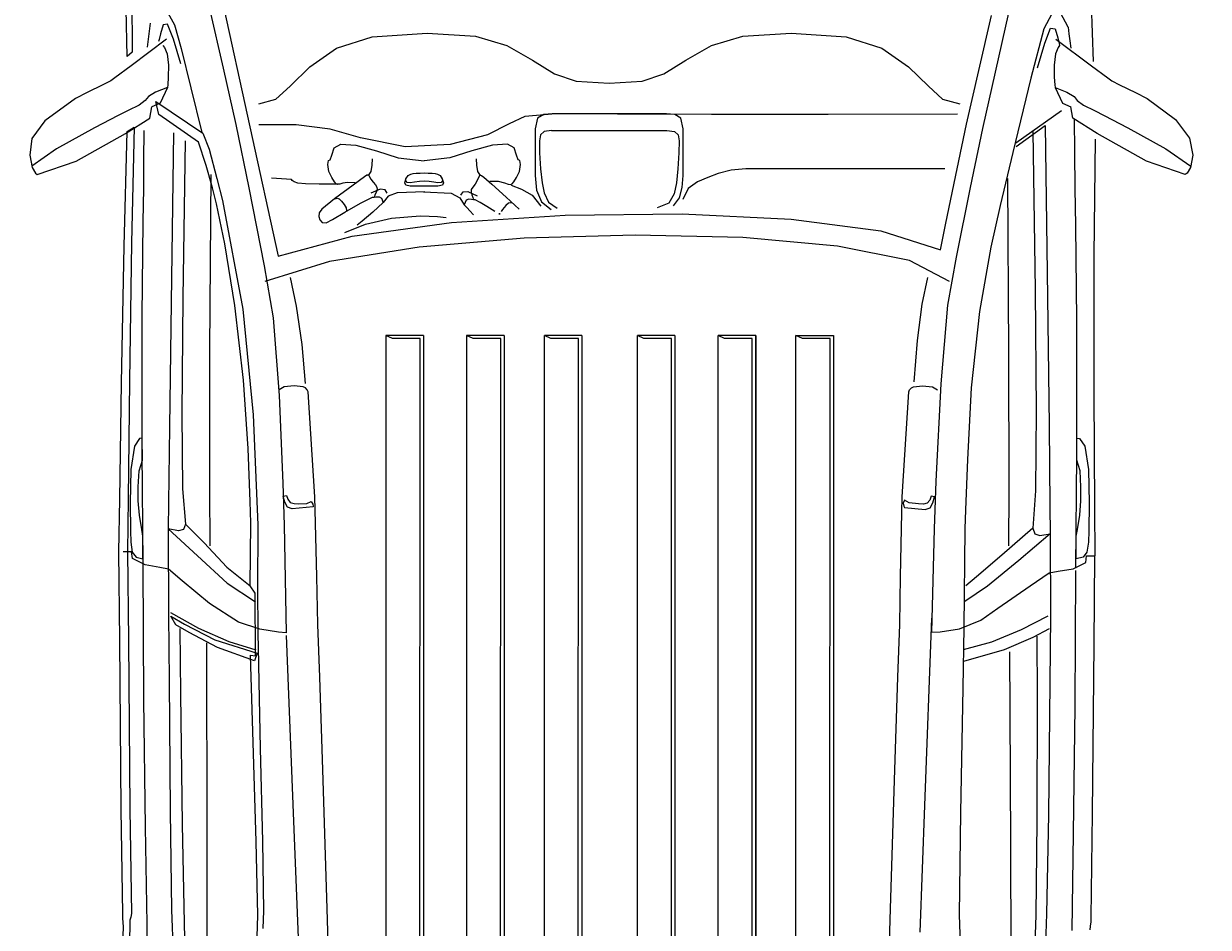
# Model space of a CAD drawing. Units: inches. Extents: x 37 to 706, y -568 to 110.
# Tile 4 of 24: x 126 to 171, y -413 to -378. Entities that reach past the tile are written whole.
import ezdxf

# ---------------------------------------------------------------- set-up
doc = ezdxf.new("R2010")
doc.units = ezdxf.units.IN
doc.header["$MEASUREMENT"] = 0
for name, color, linetype, lineweight in [('A-ANNO-DIMS', 2, 'Continuous', 18), ('A-SITE-VEHI', 8, 'Continuous', 13), ('A-WALL-PATT', 252, 'Continuous', 13)]:
    doc.layers.add(name, color=color, linetype=linetype, lineweight=lineweight)
doc.styles.get("Standard").update_dxf_attribs({"font": 'arial.ttf'})
doc.dimstyles.get("Standard").update_dxf_attribs({"dimtxt": 0.18, "dimasz": 0.18, "dimexe": 0.18, "dimexo": 0.0625, "dimgap": 0.09, "dimtad": 0, "dimtih": 1, "dimtoh": 1, "dimdec": 0, "dimzin": 0, "dimdsep": 46, "dimlunit": 3, "dimtxsty": 'Standard', "dimcen": 0.09, "dimadec": 0, "dimazin": 0, "dimtfac": 1, "dimtdec": 0, "dimtofl": 0, "dimtmove": 0, "dimatfit": 3, "dimfxl": 1, "dimtolj": 1, "dimtzin": 0, "dimarcsym": 0})

# ---------------------------------------------------------------- blocks, each defined once
blk = doc.blocks.new('CAR-SEDAN-PLAN')
for p, q in [((7.243, 63.902), (9.479, 53.69)), ((3.894, 63.679), (3.912, 61.483)), ((3.719, 61.318), (3.672, 63.126)), ((5.211, 63.093), (5.522, 62.522)), ((6.866, 63.136), (7.386, 60.866)), ((37.389, 62.984), (36.869, 60.714)), ((39.044, 62.941), (38.733, 62.37)), ((39.657, 62.441), (39.37, 62.983)), ((40.544, 63.318), (40.611, 61.119)), ((4.598, 62.593), (4.555, 62.29)), ((5.096, 62.522), (4.986, 62.183)), ((5.263, 62.546), (5.096, 62.522)), ((5.485, 61.977), (5.263, 62.546)), ((5.522, 62.522), (5.778, 61.618)), ((36.246, 60.784), (36.731, 62.877)), ((4.555, 62.29), (4.518, 61.981)), ((4.986, 62.183), (4.933, 61.962)), ((11.711, 61.631), (13.079, 62.064)), ((13.079, 62.064), (15.179, 62.211)), ((15.179, 62.211), (17.021, 62.087)), ((17.021, 62.087), (18.221, 61.732)), ((26.04, 61.732), (27.24, 62.087)), ((27.24, 62.087), (29.082, 62.211)), ((29.082, 62.211), (31.182, 62.064)), ((31.182, 62.064), (32.55, 61.631)), ((38.733, 62.37), (38.23, 60.486)), ((38.77, 61.826), (38.993, 62.394)), ((38.993, 62.394), (39.16, 62.37)), ((39.16, 62.37), (39.269, 62.031)), ((39.269, 62.031), (39.323, 61.81)), ((39.657, 62.441), (39.694, 62.178)), ((39.694, 62.178), (39.728, 61.911)), ((5.225, 61.98), (3.867, 60.965)), ((4.518, 61.981), (4.486, 61.667)), ((4.933, 61.962), (4.918, 61.883)), ((5.083, 61.731), (5.138, 61.656)), ((5.138, 61.656), (5.241, 61.415)), ((5.77, 61.03), (5.485, 61.977)), ((5.778, 61.618), (6.153, 60.123)), ((10.694, 60.923), (11.711, 61.631)), ((18.221, 61.732), (19.198, 61.17)), ((25.063, 61.17), (26.04, 61.732)), ((32.55, 61.631), (33.567, 60.923)), ((38.485, 60.879), (38.77, 61.826)), ((39.282, 61.656), (39.179, 61.415)), ((39.195, 61.98), (40.553, 60.965)), ((39.337, 61.731), (39.282, 61.656)), ((39.323, 61.81), (39.337, 61.731)), ((39.728, 61.911), (39.758, 61.639)), ((3.912, 61.483), (3.719, 61.318)), ((5.241, 61.415), (5.296, 60.985)), ((19.198, 61.17), (20.044, 60.65)), ((24.217, 60.65), (25.063, 61.17)), ((39.179, 61.415), (39.124, 60.985)), ((3.867, 60.965), (3.244, 60.496)), ((5.296, 60.985), (5.287, 60.527)), ((7.386, 60.866), (7.866, 58.722)), ((9.94, 60.179), (10.694, 60.923)), ((20.044, 60.65), (20.871, 60.374)), ((23.39, 60.374), (24.217, 60.65)), ((33.567, 60.923), (34.321, 60.179)), ((35.784, 58.735), (36.246, 60.784)), ((36.869, 60.714), (36.389, 58.57)), ((39.124, 60.985), (39.133, 60.527)), ((40.553, 60.965), (41.176, 60.496)), ((2.793, 60.236), (2.192, 59.94)), ((3.094, 60.381), (2.793, 60.236)), ((3.244, 60.496), (3.094, 60.381)), ((5.27, 60.235), (5.26, 60.133)), ((5.287, 60.527), (5.27, 60.235)), ((20.871, 60.374), (22.131, 60.293)), ((22.131, 60.293), (23.39, 60.374)), ((38.23, 60.486), (37.544, 57.648)), ((39.133, 60.527), (39.151, 60.235)), ((39.151, 60.235), (39.16, 60.133)), ((41.176, 60.496), (41.326, 60.381)), ((41.326, 60.381), (41.628, 60.236)), ((41.628, 60.236), (42.229, 59.941)), ((2.192, 59.94), (1.744, 59.706)), ((4.534, 59.788), (4.408, 59.635)), ((4.803, 59.956), (4.534, 59.788)), ((5.26, 60.133), (4.803, 59.956)), ((5.26, 60.133), (4.976, 59.529)), ((6.153, 60.123), (6.566, 58.409)), ((9.397, 59.68), (9.94, 60.179)), ((34.321, 60.179), (34.865, 59.68)), ((39.16, 60.133), (39.444, 59.529)), ((39.16, 60.133), (39.617, 59.956)), ((39.617, 59.956), (39.886, 59.788)), ((39.886, 59.788), (40.012, 59.635)), ((42.229, 59.941), (42.676, 59.706)), ((1.744, 59.706), (0.573, 58.863)), ((4.173, 59.456), (3.756, 59.246)), ((4.408, 59.635), (4.173, 59.456)), ((4.586, 58.96), (4.657, 59.387)), ((4.976, 59.529), (4.657, 59.387)), ((4.806, 59.598), (6.608, 58.388)), ((4.93, 59.103), (4.806, 59.598)), ((8.74, 59.507), (9.397, 59.68)), ((34.865, 59.68), (35.522, 59.507)), ((39.444, 59.529), (39.764, 59.387)), ((39.835, 58.96), (39.764, 59.387)), ((40.012, 59.635), (40.248, 59.456)), ((40.248, 59.456), (40.665, 59.246)), ((42.676, 59.706), (43.766, 58.903)), ((0.573, 58.863), (0.081, 58.181)), ((3.378, 59.067), (2.473, 58.595)), ((3.756, 59.246), (3.378, 59.067)), ((3.652, 58.378), (4.586, 58.96)), ((6.443, 58.044), (4.93, 59.103)), ((18.909, 59.028), (18.306, 58.744)), ((20.089, 59.124), (18.909, 59.028)), ((19.397, 58.963), (19.308, 58.556)), ((19.628, 59.105), (19.397, 58.963)), ((19.948, 59.122), (19.628, 59.105)), ((24.314, 59.122), (19.948, 59.122)), ((22.452, 59.111), (20.089, 59.124)), ((26.04, 59.104), (22.452, 59.111)), ((24.634, 59.105), (24.314, 59.122)), ((24.864, 58.963), (24.634, 59.105)), ((24.953, 58.556), (24.864, 58.963)), ((30.49, 59.105), (26.04, 59.104)), ((35.437, 59.117), (30.49, 59.105)), ((39.408, 59.245), (37.668, 58.002)), ((40.768, 58.378), (39.835, 58.96)), ((39.893, 58.942), (39.907, 57.649)), ((40.665, 59.246), (41.042, 59.067)), ((41.042, 59.067), (41.947, 58.595)), ((43.766, 58.903), (44.299, 58.201)), ((2.473, 58.595), (1.023, 57.787)), ((1.762, 57.317), (3.652, 58.378)), ((3.605, 54.068), (3.719, 58.456)), ((3.719, 58.456), (3.98, 58.613)), ((3.98, 58.613), (3.877, 54.201)), ((4.349, 58.487), (4.338, 57.349)), ((5.491, 58.398), (5.4, 51.914)), ((6.608, 58.388), (6.849, 57.774)), ((7.866, 58.722), (8.367, 56.297)), ((10.166, 58.704), (8.741, 58.704)), ((11.465, 58.539), (10.166, 58.704)), ((12.633, 58.209), (11.465, 58.539)), ((18.306, 58.744), (17.476, 58.319)), ((19.308, 58.556), (19.308, 56.766)), ((19.642, 58.446), (19.501, 58.322)), ((19.929, 58.483), (19.642, 58.446)), ((19.929, 58.483), (24.332, 58.483)), ((24.332, 58.483), (24.619, 58.446)), ((24.619, 58.446), (24.76, 58.322)), ((24.953, 56.766), (24.953, 58.556)), ((35.422, 57.018), (35.784, 58.735)), ((36.389, 58.57), (35.918, 56.312)), ((37.675, 57.879), (38.788, 58.684)), ((38.307, 58.463), (38.397, 52.383)), ((38.788, 58.684), (38.877, 52.125)), ((42.658, 57.317), (40.768, 58.378)), ((41.947, 58.595), (43.397, 57.787)), ((0.081, 58.181), (0, 57.551)), ((5.932, 58.096), (5.844, 52.097)), ((6.733, 57.156), (6.443, 58.044)), ((11.627, 57.82), (11.874, 57.964)), ((11.874, 57.964), (12.448, 57.926)), ((12.448, 57.926), (13.235, 57.705)), ((14.34, 57.866), (12.633, 58.209)), ((16.051, 57.949), (14.34, 57.866)), ((17.476, 58.319), (16.051, 57.949)), ((17.673, 57.926), (16.886, 57.705)), ((18.247, 57.964), (17.673, 57.926)), ((18.494, 57.82), (18.247, 57.964)), ((19.501, 58.322), (19.463, 58.09)), ((19.463, 58.09), (19.473, 57.639)), ((24.76, 58.322), (24.798, 58.09)), ((24.798, 58.09), (24.788, 57.639)), ((40.697, 58.154), (40.647, 53.716)), ((44.299, 58.201), (44.42, 57.551)), ((0, 57.551), (0.089, 57.074)), ((1.023, 57.787), (0.071, 57.125)), ((6.849, 57.774), (7.147, 56.658)), ((11.466, 57.369), (11.535, 57.542)), ((11.535, 57.542), (11.627, 57.82)), ((13.235, 57.705), (14.073, 57.447)), ((16.886, 57.705), (16.048, 57.447)), ((18.587, 57.542), (18.494, 57.82)), ((18.655, 57.369), (18.587, 57.542)), ((19.473, 57.639), (19.505, 57.028)), ((24.788, 57.639), (24.756, 57.028)), ((37.544, 57.648), (37.064, 55.622)), ((39.907, 57.649), (39.918, 56.282)), ((43.397, 57.787), (44.349, 57.125)), ((44.42, 57.551), (44.331, 57.074)), ((0.089, 57.074), (0.218, 56.857)), ((0.284, 56.806), (1.762, 57.317)), ((4.338, 57.349), (4.334, 56.285)), ((6.975, 56.299), (6.733, 57.156)), ((11.38, 57.195), (11.412, 57.338)), ((11.422, 56.921), (11.38, 57.195)), ((11.412, 57.338), (11.466, 57.369)), ((13.059, 57.159), (13.022, 56.924)), ((13.069, 57.405), (13.059, 57.159)), ((14.073, 57.447), (15.061, 57.323)), ((16.048, 57.447), (15.061, 57.323)), ((17.052, 57.405), (17.064, 57.16)), ((17.064, 57.16), (17.104, 56.925)), ((18.71, 57.338), (18.655, 57.369)), ((18.7, 56.921), (18.742, 57.195)), ((18.742, 57.195), (18.71, 57.338)), ((19.505, 57.028), (19.564, 56.492)), ((24.756, 57.028), (24.697, 56.492)), ((27.353, 57.026), (26.785, 56.971)), ((34.947, 57.026), (27.353, 57.026)), ((34.991, 54.942), (35.422, 57.018)), ((44.136, 56.806), (42.658, 57.317)), ((44.331, 57.074), (44.202, 56.857)), ((0.218, 56.857), (0.284, 56.806)), ((6.907, 56.804), (6.866, 50.096)), ((7.147, 56.658), (7.352, 55.813)), ((9.992, 56.613), (9.236, 56.668)), ((10.013, 56.583), (9.992, 56.613)), ((10.09, 56.523), (10.013, 56.583)), ((11.533, 56.687), (11.422, 56.921)), ((11.635, 56.528), (11.533, 56.687)), ((12.786, 56.72), (12.355, 56.402)), ((12.875, 56.778), (12.786, 56.72)), ((12.911, 56.779), (12.875, 56.778)), ((12.917, 56.768), (12.911, 56.779)), ((13.022, 56.924), (12.917, 56.768)), ((12.953, 56.766), (13.019, 56.626)), ((13.019, 56.626), (13.109, 56.514)), ((14.318, 56.49), (14.367, 56.638)), ((14.36, 56.563), (14.367, 56.638)), ((14.367, 56.638), (14.454, 56.763)), ((14.454, 56.763), (14.547, 56.817)), ((14.547, 56.817), (14.641, 56.839)), ((14.641, 56.839), (14.756, 56.854)), ((14.756, 56.854), (14.903, 56.863)), ((14.903, 56.863), (15.061, 56.866)), ((15.061, 56.866), (15.218, 56.863)), ((15.218, 56.863), (15.366, 56.854)), ((15.366, 56.854), (15.481, 56.839)), ((15.481, 56.839), (15.574, 56.817)), ((15.574, 56.817), (15.668, 56.763)), ((15.668, 56.763), (15.755, 56.638)), ((15.755, 56.638), (15.804, 56.49)), ((15.755, 56.638), (15.761, 56.563)), ((17.103, 56.601), (17.016, 56.44)), ((17.171, 56.766), (17.103, 56.601)), ((17.104, 56.925), (17.207, 56.766)), ((17.207, 56.766), (17.214, 56.776)), ((17.214, 56.776), (17.249, 56.774)), ((17.249, 56.774), (17.335, 56.711)), ((17.335, 56.711), (17.648, 56.433)), ((18.486, 56.528), (18.589, 56.687)), ((18.589, 56.687), (18.7, 56.921)), ((19.308, 56.766), (19.356, 56.213)), ((24.923, 56.308), (24.953, 56.766)), ((25.895, 56.696), (25.508, 56.53)), ((26.297, 56.842), (25.895, 56.696)), ((26.785, 56.971), (26.297, 56.842)), ((37.348, 56.652), (37.389, 49.984)), ((44.202, 56.857), (44.136, 56.806)), ((4.334, 56.285), (4.314, 54.993)), ((7.131, 55.691), (6.975, 56.299)), ((8.367, 56.297), (8.95, 53.318)), ((10.24, 56.475), (10.09, 56.523)), ((10.531, 56.453), (10.24, 56.475)), ((11.052, 56.441), (10.531, 56.453)), ((11.845, 56.437), (11.052, 56.441)), ((11.702, 56.448), (11.635, 56.528)), ((12.355, 56.402), (11.642, 55.878)), ((11.766, 56.42), (11.702, 56.448)), ((11.845, 56.437), (11.766, 56.42)), ((11.958, 56.473), (11.845, 56.437)), ((12.138, 56.495), (11.958, 56.473)), ((12.421, 56.483), (12.138, 56.495)), ((13.382, 56.251), (13.02, 56.096)), ((13.109, 56.514), (13.201, 56.416)), ((13.223, 56.122), (13.181, 56.026)), ((13.201, 56.416), (13.259, 56.323)), ((13.263, 56.228), (13.223, 56.122)), ((13.259, 56.323), (13.263, 56.228)), ((13.569, 56.226), (13.382, 56.251)), ((13.642, 56.091), (13.569, 56.226)), ((15.088, 56.145), (14.025, 56.105)), ((14.36, 56.396), (14.318, 56.49)), ((14.415, 56.496), (14.36, 56.563)), ((14.531, 56.364), (14.36, 56.396)), ((14.531, 56.483), (14.415, 56.496)), ((14.697, 56.511), (14.531, 56.483)), ((15.59, 56.364), (14.531, 56.364)), ((14.885, 56.536), (14.697, 56.511)), ((15.07, 56.547), (14.885, 56.536)), ((15.033, 56.145), (16.092, 56.088)), ((15.249, 56.536), (15.07, 56.547)), ((15.429, 56.511), (15.249, 56.536)), ((15.59, 56.483), (15.429, 56.511)), ((15.706, 56.496), (15.59, 56.483)), ((15.761, 56.396), (15.59, 56.364)), ((15.761, 56.563), (15.706, 56.496)), ((15.804, 56.49), (15.761, 56.396)), ((16.467, 56.017), (16.547, 56.148)), ((16.547, 56.148), (16.735, 56.163)), ((16.735, 56.163), (17.089, 55.989)), ((16.862, 56.228), (16.852, 56.134)), ((16.852, 56.134), (16.887, 56.026)), ((16.924, 56.318), (16.862, 56.228)), ((17.016, 56.44), (16.924, 56.318)), ((17.573, 56.556), (17.889, 56.549)), ((17.648, 56.433), (18.193, 55.945)), ((17.889, 56.549), (18.13, 56.492)), ((18.13, 56.492), (18.276, 56.437)), ((18.276, 56.437), (18.355, 56.42)), ((18.355, 56.42), (18.419, 56.448)), ((18.383, 56.393), (18.78, 56.247)), ((18.419, 56.448), (18.486, 56.528)), ((18.78, 56.247), (19.189, 56.016)), ((19.356, 56.213), (19.539, 55.764)), ((19.564, 56.492), (19.646, 56.107)), ((24.697, 56.492), (24.611, 56.07)), ((24.809, 55.915), (24.923, 56.308)), ((25.149, 56.27), (24.945, 55.856)), ((25.508, 56.53), (25.149, 56.27)), ((35.918, 56.312), (35.385, 53.644)), ((39.918, 56.282), (39.941, 54.841)), ((7.449, 54.154), (7.131, 55.691)), ((7.352, 55.813), (8.134, 51.663)), ((11.642, 55.878), (11.149, 55.48)), ((11.673, 55.883), (11.744, 55.903)), ((11.744, 55.903), (11.817, 55.879)), ((11.817, 55.879), (11.906, 55.788)), ((11.906, 55.788), (12.007, 55.658)), ((12.025, 55.371), (12.63, 55.707)), ((12.63, 55.707), (13.094, 55.946)), ((13.094, 55.946), (13.107, 55.941)), ((13.495, 55.733), (13.1, 55.373)), ((13.107, 55.941), (13.151, 55.937)), ((13.151, 55.937), (13.232, 55.948)), ((13.181, 56.026), (13.168, 55.97)), ((13.168, 55.97), (13.168, 55.951)), ((13.232, 55.948), (13.338, 55.959)), ((13.338, 55.959), (13.435, 55.908)), ((13.435, 55.908), (13.495, 55.733)), ((13.686, 55.974), (13.495, 55.733)), ((14.025, 56.105), (13.686, 55.974)), ((16.092, 56.088), (16.42, 55.921)), ((16.42, 55.921), (16.595, 55.651)), ((16.664, 55.823), (16.595, 55.651)), ((16.764, 55.869), (16.664, 55.823)), ((16.869, 55.852), (16.764, 55.869)), ((16.949, 55.838), (16.869, 55.852)), ((16.887, 56.026), (16.924, 55.928)), ((16.924, 55.928), (16.933, 55.871)), ((16.933, 55.871), (16.933, 55.852)), ((16.993, 55.84), (16.949, 55.838)), ((17.006, 55.843), (16.993, 55.84)), ((17.202, 55.734), (17.006, 55.843)), ((17.461, 55.581), (17.202, 55.734)), ((18.279, 55.71), (18.185, 55.624)), ((18.193, 55.945), (18.694, 55.483)), ((18.352, 55.729), (18.279, 55.71)), ((18.422, 55.706), (18.352, 55.729)), ((19.189, 56.016), (19.512, 55.595)), ((19.539, 55.764), (19.916, 55.467)), ((19.646, 56.107), (19.813, 55.756)), ((19.813, 55.756), (20.146, 55.524)), ((24.411, 55.715), (23.966, 55.531)), ((24.611, 56.07), (24.411, 55.715)), ((24.58, 55.614), (24.809, 55.915)), ((11.052, 55.336), (11.032, 55.197)), ((11.149, 55.48), (11.052, 55.336)), ((11.558, 55.084), (12.025, 55.371)), ((12.007, 55.658), (12.081, 55.535)), ((12.081, 55.535), (12.097, 55.422)), ((13.1, 55.373), (12.692, 55.023)), ((13.811, 55.137), (14.905, 55.222)), ((14.905, 55.222), (15.259, 55.221)), ((15.259, 55.221), (15.572, 55.208)), ((15.572, 55.208), (15.9, 55.17)), ((16.11, 54.971), (20.454, 55.259)), ((16.595, 55.651), (16.702, 55.534)), ((16.702, 55.534), (16.812, 55.413)), ((16.812, 55.413), (16.943, 55.271)), ((17.765, 55.393), (17.461, 55.581)), ((17.911, 55.307), (17.963, 55.31)), ((17.928, 55.308), (17.911, 55.307)), ((17.945, 55.309), (17.928, 55.308)), ((17.963, 55.31), (17.945, 55.309)), ((18.053, 55.468), (18.004, 55.394)), ((18.116, 55.545), (18.053, 55.468)), ((18.185, 55.624), (18.116, 55.545)), ((20.454, 55.259), (24.918, 55.306)), ((24.918, 55.306), (29.077, 55.104)), ((37.064, 55.622), (36.708, 54.03)), ((4.314, 54.993), (4.274, 51.392)), ((11.032, 55.197), (11.073, 55.073)), ((11.073, 55.073), (11.161, 54.978)), ((11.161, 54.978), (11.312, 54.961)), ((11.312, 54.961), (11.558, 55.084)), ((12.03, 54.597), (12.826, 54.914)), ((12.31, 54.446), (16.11, 54.971)), ((12.692, 55.023), (12.503, 54.866)), ((12.826, 54.914), (13.811, 55.137)), ((29.077, 55.104), (32.507, 54.649)), ((34.783, 53.934), (34.991, 54.942)), ((39.941, 54.841), (39.982, 51.24)), ((9.479, 53.69), (12.31, 54.446)), ((18.887, 54.369), (14.875, 54.03)), ((23.128, 54.492), (18.887, 54.369)), ((27.235, 54.394), (23.128, 54.492)), ((30.846, 54.07), (27.235, 54.394)), ((32.507, 54.649), (34.783, 53.934)), ((3.505, 48.842), (3.605, 54.068)), ((3.877, 54.201), (3.8, 48.921)), ((7.831, 51.803), (7.449, 54.154)), ((14.875, 54.03), (11.451, 53.479)), ((33.599, 53.515), (30.846, 54.07)), ((36.708, 54.03), (36.272, 51.578)), ((11.451, 53.479), (8.979, 52.723)), ((35.133, 52.723), (33.599, 53.515)), ((35.385, 53.644), (35.049, 51.82)), ((40.647, 53.716), (40.649, 48.459)), ((8.95, 53.318), (9.297, 51.325)), ((9.937, 52.871), (10.178, 51.78)), ((34.292, 52.871), (34.07, 51.849)), ((5.844, 52.097), (5.807, 47.67)), ((38.397, 52.383), (38.441, 47.777)), ((38.877, 52.125), (38.933, 47.216)), ((5.4, 51.914), (5.336, 47.171)), ((8.162, 48.95), (7.831, 51.803)), ((8.134, 51.663), (8.527, 47.62)), ((10.178, 51.78), (10.383, 50.312)), ((34.07, 51.849), (33.895, 50.463)), ((35.049, 51.82), (34.796, 48.812)), ((4.274, 51.392), (4.272, 47.831)), ((9.297, 51.325), (9.518, 48.368)), ((36.272, 51.578), (35.963, 48.661)), ((39.982, 51.24), (39.983, 47.679)), ((10.383, 50.312), (10.515, 48.827)), ((13.846, 50.543), (13.603, 50.661)), ((15.035, 50.661), (13.603, 50.661)), ((13.604, 13.133), (13.604, 50.661)), ((14.905, 50.543), (13.846, 50.543)), ((14.891, 13.73), (14.905, 50.543)), ((15.034, 50.661), (15.034, 13.133)), ((15.035, 50.661), (15.035, 13.133)), ((16.928, 50.543), (16.685, 50.661)), ((18.117, 50.661), (16.685, 50.661)), ((16.686, 13.133), (16.686, 50.661)), ((17.987, 50.543), (16.928, 50.543)), ((17.973, 13.73), (17.987, 50.543)), ((18.115, 50.661), (18.115, 13.133)), ((18.117, 50.661), (18.117, 13.133)), ((19.899, 50.543), (19.656, 50.661)), ((21.088, 50.661), (19.656, 50.661)), ((19.657, 13.133), (19.657, 50.661)), ((20.958, 50.543), (19.899, 50.543)), ((20.944, 13.73), (20.958, 50.543)), ((21.087, 50.661), (21.087, 13.133)), ((21.088, 50.661), (21.088, 13.133)), ((23.454, 50.543), (23.211, 50.661)), ((24.643, 50.661), (23.211, 50.661)), ((23.212, 13.133), (23.212, 50.661)), ((24.513, 50.543), (23.454, 50.543)), ((24.499, 13.73), (24.513, 50.543)), ((24.642, 50.661), (24.642, 13.133)), ((24.643, 50.661), (24.643, 13.133)), ((26.535, 50.543), (26.293, 50.661)), ((27.725, 50.661), (26.293, 50.661)), ((26.294, 13.133), (26.294, 50.661)), ((27.595, 50.543), (26.535, 50.543)), ((27.581, 13.73), (27.595, 50.543)), ((27.723, 50.661), (27.723, 13.133)), ((27.725, 50.661), (27.725, 13.133)), ((29.265, 13.133), (29.265, 50.661)), ((29.508, 50.543), (29.265, 50.661)), ((29.265, 50.661), (30.696, 50.661)), ((30.567, 50.543), (29.508, 50.543)), ((30.553, 13.73), (30.567, 50.543)), ((30.696, 50.661), (30.696, 13.133)), ((33.895, 50.463), (33.764, 48.882)), ((6.866, 50.096), (6.863, 44.784)), ((37.389, 49.984), (37.39, 44.744)), ((3.8, 48.921), (3.752, 44.431)), ((8.341, 46.338), (8.162, 48.95)), ((3.432, 44.406), (3.505, 48.842)), ((9.72, 48.689), (9.523, 48.579)), ((10.096, 48.73), (9.72, 48.689)), ((10.436, 48.697), (10.096, 48.73)), ((10.523, 48.654), (10.436, 48.697)), ((10.593, 48.583), (10.523, 48.654)), ((10.625, 48.497), (10.593, 48.583)), ((10.882, 44.496), (10.625, 48.497)), ((33.322, 44.496), (33.571, 48.497)), ((33.571, 48.497), (33.602, 48.583)), ((33.602, 48.583), (33.672, 48.654)), ((33.672, 48.654), (33.759, 48.697)), ((33.759, 48.697), (34.099, 48.73)), ((34.099, 48.73), (34.475, 48.689)), ((34.475, 48.689), (34.672, 48.579)), ((34.796, 48.812), (34.613, 45.086)), ((35.963, 48.661), (35.82, 45.919)), ((40.649, 48.459), (40.673, 44.07)), ((9.518, 48.368), (9.661, 45.012)), ((4.272, 47.831), (4.279, 46.22)), ((5.807, 47.67), (5.836, 44.794)), ((8.527, 47.62), (8.706, 43.417)), ((38.441, 47.777), (38.417, 44.723)), ((39.983, 47.679), (39.977, 46.068)), ((5.336, 47.171), (5.299, 44.26)), ((38.933, 47.216), (38.963, 44.139)), ((4.192, 46.715), (3.994, 46.427)), ((4.293, 46.735), (4.192, 46.715)), ((4.301, 45.897), (4.293, 46.735)), ((39.989, 45.897), (39.997, 46.735)), ((39.997, 46.735), (40.098, 46.715)), ((40.098, 46.715), (40.296, 46.427)), ((3.994, 46.427), (3.854, 45.534)), ((4.279, 46.22), (4.314, 41.922)), ((8.42, 44.315), (8.341, 46.338)), ((40.296, 46.427), (40.436, 45.534)), ((4.174, 45.486), (4.301, 45.897)), ((35.82, 45.919), (35.739, 43.991)), ((39.977, 46.068), (39.941, 41.77)), ((40.115, 45.486), (39.989, 45.897)), ((3.854, 45.534), (3.83, 44.25)), ((4.14, 44.879), (4.174, 45.486)), ((40.15, 44.879), (40.115, 45.486)), ((40.436, 45.534), (40.46, 44.25)), ((4.141, 44.332), (4.14, 44.879)), ((9.661, 45.012), (9.713, 43.414)), ((34.613, 45.086), (34.542, 43.262)), ((40.149, 44.332), (40.15, 44.879)), ((3.403, 42.392), (3.432, 44.406)), ((3.752, 44.431), (3.734, 42.392)), ((5.836, 44.794), (5.948, 43.449)), ((6.863, 44.784), (6.869, 42.622)), ((9.676, 44.516), (9.798, 44.542)), ((9.733, 44.29), (9.676, 44.516)), ((9.798, 44.542), (9.85, 44.396)), ((9.85, 44.396), (9.949, 44.274)), ((10.962, 41.449), (10.882, 44.496)), ((33.258, 41.449), (33.322, 44.496)), ((33.404, 44.362), (33.363, 44.248)), ((33.591, 44.267), (33.404, 44.362)), ((34.379, 44.368), (34.28, 44.247)), ((34.431, 44.514), (34.379, 44.368)), ((34.554, 44.489), (34.431, 44.514)), ((34.496, 44.262), (34.554, 44.489)), ((37.39, 44.744), (37.384, 42.623)), ((38.417, 44.723), (38.307, 43.297)), ((3.83, 44.25), (3.844, 43.196)), ((4.188, 43.792), (4.141, 44.332)), ((5.299, 44.26), (5.287, 43.269)), ((8.437, 43.503), (8.42, 44.315)), ((9.838, 44.098), (9.733, 44.29)), ((10.025, 44.031), (9.838, 44.098)), ((9.949, 44.274), (10.095, 44.234)), ((10.824, 44.11), (10.025, 44.031)), ((10.095, 44.234), (10.264, 44.226)), ((10.264, 44.226), (10.577, 44.234)), ((10.577, 44.234), (10.743, 44.307)), ((10.743, 44.307), (10.805, 44.214)), ((10.805, 44.214), (10.824, 44.14)), ((10.824, 44.14), (10.824, 44.11)), ((33.363, 44.248), (33.384, 44.134)), ((33.384, 44.134), (33.405, 44.082)), ((33.405, 44.082), (34.204, 44.004)), ((33.943, 44.22), (33.591, 44.267)), ((34.134, 44.207), (33.943, 44.22)), ((34.28, 44.247), (34.134, 44.207)), ((34.204, 44.004), (34.391, 44.071)), ((34.391, 44.071), (34.496, 44.262)), ((35.739, 43.991), (35.714, 43.262)), ((38.963, 44.139), (38.971, 43.074)), ((40.102, 43.792), (40.149, 44.332)), ((40.46, 44.25), (40.446, 43.196)), ((40.673, 44.07), (40.687, 42.232)), ((4.273, 43.24), (4.188, 43.792)), ((5.948, 43.449), (5.871, 43.237)), ((5.948, 43.449), (6.66, 42.737)), ((8.416, 41.085), (8.437, 43.503)), ((40.017, 43.24), (40.102, 43.792)), ((3.844, 43.196), (3.857, 42.759)), ((4.32, 42.987), (4.273, 43.24)), ((5.287, 43.269), (6.407, 42.232)), ((5.672, 43.197), (5.287, 43.269)), ((5.287, 43.269), (5.301, 39.967)), ((5.871, 43.237), (5.672, 43.197)), ((8.706, 43.417), (8.689, 40.947)), ((9.713, 43.414), (9.796, 39.289)), ((34.542, 43.262), (34.438, 39.318)), ((35.714, 43.262), (35.681, 39.496)), ((38.307, 43.297), (37.13, 42.261)), ((38.971, 43.074), (37.772, 42.057)), ((38.307, 43.297), (38.385, 43.074)), ((38.385, 43.074), (38.586, 43.013)), ((38.586, 43.013), (38.971, 43.074)), ((38.971, 43.074), (38.982, 39.925)), ((39.97, 42.987), (40.017, 43.24)), ((40.446, 43.196), (40.433, 42.759)), ((3.857, 42.759), (3.913, 42.374)), ((4.32, 42.116), (4.32, 42.987)), ((6.66, 42.737), (7.526, 41.803)), ((39.97, 42.116), (39.97, 42.987)), ((40.433, 42.759), (40.377, 42.374)), ((3.432, 39.004), (3.403, 42.392)), ((3.888, 42.384), (3.568, 42.392)), ((3.734, 42.392), (3.762, 39.007)), ((3.924, 42.135), (3.888, 42.384)), ((3.913, 42.374), (4.061, 42.185)), ((4.399, 41.888), (3.924, 42.135)), ((4.061, 42.185), (4.32, 42.116)), ((6.407, 42.232), (7.533, 41.191)), ((37.13, 42.261), (36.157, 41.433)), ((40.229, 42.185), (39.97, 42.116)), ((40.377, 42.374), (40.229, 42.185)), ((40.332, 41.983), (40.367, 42.232)), ((40.367, 42.232), (40.674, 42.232)), ((40.658, 38.847), (40.687, 42.232)), ((4.314, 41.922), (4.342, 36.731)), ((4.968, 41.787), (4.399, 41.888)), ((5.301, 41.728), (4.968, 41.787)), ((5.819, 41.275), (5.301, 41.728)), ((7.526, 41.803), (8.416, 41.085)), ((37.772, 42.057), (36.584, 41.081)), ((38.936, 41.591), (39.274, 41.645)), ((39.274, 41.645), (39.851, 41.74)), ((39.851, 41.74), (40.332, 41.983)), ((39.946, 41.674), (39.918, 36.482)), ((6.86, 40.42), (5.819, 41.275)), ((7.533, 41.191), (8.616, 40.477)), ((10.998, 39.61), (10.962, 41.449)), ((33.232, 39.61), (33.258, 41.449)), ((36.157, 41.433), (35.752, 41.094)), ((38.211, 41.09), (38.936, 41.591)), ((8.61, 40.812), (8.416, 41.085)), ((8.623, 38.413), (8.61, 40.812)), ((8.689, 40.947), (8.707, 39.376)), ((36.584, 41.081), (35.717, 40.49)), ((36.975, 40.234), (38.211, 41.09)), ((7.97, 39.706), (6.86, 40.42)), ((5.301, 39.967), (5.315, 37.467)), ((5.378, 40.068), (6.446, 39.47)), ((5.576, 39.596), (5.383, 39.926)), ((5.383, 39.926), (5.907, 39.624)), ((34.436, 39.852), (34.17, 32.694)), ((36.321, 39.78), (36.975, 40.234)), ((38.884, 39.936), (37.863, 39.414)), ((38.982, 39.925), (38.961, 37.396)), ((6.083, 39.306), (5.576, 39.596)), ((5.727, 39.459), (5.754, 36.963)), ((5.907, 39.624), (7.068, 39.031)), ((6.446, 39.47), (7.6, 38.961)), ((8.786, 39.439), (7.97, 39.706)), ((8.707, 39.376), (8.71, 39.215)), ((9.493, 39.318), (8.786, 39.439)), ((11.071, 37.604), (10.998, 39.61)), ((33.159, 37.604), (33.232, 39.61)), ((34.768, 39.333), (35.515, 39.45)), ((35.515, 39.45), (36.321, 39.78)), ((35.681, 39.496), (35.635, 37.18)), ((37.863, 39.414), (36.73, 38.932)), ((38.331, 39.125), (38.947, 39.462)), ((3.493, 32.542), (3.432, 39.004)), ((3.762, 39.007), (3.823, 32.551)), ((7.162, 38.735), (6.083, 39.306)), ((7.068, 39.031), (8.678, 38.516)), ((7.6, 38.961), (8.63, 38.647)), ((8.71, 39.215), (8.718, 38.766)), ((9.796, 39.289), (9.493, 39.318)), ((9.785, 39.195), (10.065, 32.102)), ((34.438, 39.318), (34.768, 39.333)), ((36.73, 38.932), (35.646, 38.643)), ((37.235, 38.651), (38.331, 39.125)), ((38.468, 39.17), (38.473, 36.823)), ((6.745, 38.908), (6.755, 31.469)), ((8.583, 38.221), (7.162, 38.735)), ((8.678, 38.516), (8.583, 38.221)), ((8.718, 38.766), (8.731, 38.071)), ((35.681, 38.217), (37.235, 38.651)), ((37.423, 38.564), (37.433, 36.292)), ((40.598, 32.392), (40.658, 38.847)), ((8.528, 35.109), (8.424, 38.44)), ((8.424, 38.44), (8.623, 38.413)), ((8.731, 38.071), (8.801, 34.877)), ((11.199, 33.662), (11.071, 37.604)), ((33.03, 33.662), (33.159, 37.604)), ((5.315, 37.467), (5.354, 32.465)), ((35.635, 37.18), (35.548, 32.425)), ((38.961, 37.396), (38.908, 32.341)), ((4.342, 36.731), (4.403, 31.875)), ((5.754, 36.963), (5.818, 31.97)), ((38.473, 36.823), (38.469, 32.105)), ((37.433, 36.292), (37.457, 31.221)), ((39.918, 36.482), (39.857, 31.627)), ((8.645, 31.317), (8.528, 35.109)), ((8.801, 34.877), (8.881, 31.335)), ((11.355, 28.753), (11.199, 33.662)), ((32.874, 28.753), (33.03, 33.662)), ((34.17, 32.694), (34.002, 27.855)), ((3.546, 28.561), (3.493, 32.542)), ((3.823, 32.551), (3.876, 28.574)), ((5.354, 32.465), (5.415, 28.71)), ((35.548, 32.425), (35.501, 28.522)), ((38.908, 32.341), (38.84, 28.558)), ((40.545, 28.416), (40.598, 32.392)), ((4.403, 31.875), (4.464, 28.172)), ((5.818, 31.97), (5.892, 28.219)), ((10.065, 32.102), (10.25, 27.635)), ((38.469, 32.105), (38.427, 28.503)), ((6.755, 31.469), (6.762, 26.153)), ((8.713, 28.508), (8.645, 31.317)), ((8.881, 31.335), (8.919, 28.667)), ((39.857, 31.627), (39.796, 27.924)), ((37.457, 31.221), (37.48, 25.971)), ((3.551, 28.393), (3.546, 28.561)), ((3.876, 28.574), (3.856, 28.436)), ((5.415, 28.71), (5.486, 26.554)), ((8.919, 28.667), (8.894, 27.992)), ((11.511, 23.847), (11.355, 28.753)), ((32.718, 23.847), (32.874, 28.753)), ((35.501, 28.522), (35.566, 26.682)), ((38.84, 28.558), (38.769, 26.402)), ((3.52, 26.505), (3.579, 28.059)), ((3.558, 28.225), (3.551, 28.393)), ((3.579, 28.059), (3.558, 28.225)), ((3.815, 28.178), (3.801, 27.531)), ((3.819, 28.315), (3.815, 28.178)), ((3.856, 28.436), (3.819, 28.315)), ((4.464, 28.172), (4.492, 26.437)), ((5.892, 28.219), (5.946, 25.954)), ((8.671, 27.267), (8.713, 28.508)), ((38.427, 28.503), (38.356, 26.347)), ((40.498, 27.951), (40.519, 28.091)), ((40.519, 28.091), (40.535, 28.246)), ((40.535, 28.246), (40.545, 28.416))]:
    blk.add_line(p, q)
blk = doc.blocks.new('*D29')
at = {"layer": 'A-ANNO-DIMS', "color": 0, "lineweight": -2, "transparency": 16777216}
for p, q in [((170.913, -348.62), (184.856, -348.62)), ((184.676, -348.8), (184.676, -394.522)), ((184.676, -440.609), (184.676, -394.888)), ((170.913, -440.789), (184.856, -440.789))]:
    blk.add_line(p, q, dxfattribs=at)
at = {"layer": 'A-ANNO-DIMS', "color": 0, "transparency": 16777216}
for points in [[(184.646, -348.8), (184.706, -348.8), (184.676, -348.62)], [(184.646, -440.609), (184.706, -440.609), (184.676, -440.789)]]:
    blk.add_solid(points, dxfattribs=at)
at = {"layer": 'Defpoints', "color": 0, "transparency": 16777216}
for p in [(170.851, -348.62), (184.676, -348.62), (170.851, -440.789)]:
    blk.add_point(p, dxfattribs=at)
at = {"layer": 'A-ANNO-DIMS', "color": 0, "transparency": 16777216, "insert": (184.676, -394.705), "char_height": 0.18, "attachment_point": 5}
blk.add_mtext('\\A1;CAR 7\'-8" TYP.', dxfattribs=at)

msp = doc.modelspace()

# ---------------------------------------------------------------- hatches: boundary and pattern name
at = {"layer": 'A-WALL-PATT'}
h = msp.add_hatch(color=256, dxfattribs=at)
h.dxf.hatch_style = 1
h.paths.add_polyline_path([(220.958, -351.708), (211.958, -351.708), (211.958, -513.708), (254.958, -513.708), (254.958, -504.708), (220.958, -504.708)], flags=17)
h.paths.add_polyline_path([(220.958, -294.708), (211.958, -294.708), (211.958, -303.708), (220.958, -303.708)], flags=17)
h.paths.add_polyline_path([(175.958, -294.708), (155.871, -294.708), (155.871, -303.708), (155.958, -303.708), (175.958, -303.708)], flags=17)
h.paths.add_polyline_path([(220.958, -16.708), (211.958, -16.708), (211.958, -142.708), (220.958, -142.708)], flags=17)
h.paths.add_polyline_path([(357.958, 51.292), (78.958, 51.292), (78.958, -513.708), (87.958, -513.708), (87.958, -303.708), (95.871, -303.708), (95.871, -294.708), (87.958, -294.708), (87.958, -142.708), (187.958, -142.708), (187.958, -133.708), (87.958, -133.708), (87.958, -25.708), (106.958, -25.708), (106.958, -16.708), (87.958, -16.708), (87.958, 42.292), (348.958, 42.292), (348.958, 17.129), (348.958, -133.708), (246.958, -133.708), (246.958, -142.708), (348.958, -142.708), (348.958, -294.708), (251.958, -294.708), (251.958, -303.708), (348.958, -303.708), (348.958, -351.708), (260.958, -351.708), (260.958, -329.708), (251.958, -329.708), (251.958, -360.708), (327.446, -360.708), (348.958, -360.708), (348.958, -504.708), (314.958, -504.708), (314.958, -513.708), (357.958, -513.708)])
h.paths.add_polyline_path([(416.958, -303.708), (402.958, -303.708), (402.958, -151.708), (478.958, -151.708), (478.958, -142.708), (402.958, -142.708), (402.958, -22.708), (409.958, -22.708), (409.958, -13.708), (402.958, -13.708), (402.958, 42.292), (663.958, 42.292), (663.958, -303.708), (566.958, -303.708), (566.958, -312.708), (663.958, -312.708), (663.958, -360.708), (575.958, -360.708), (575.958, -338.708), (566.958, -338.708), (566.958, -360.708), (566.958, -369.708), (642.446, -369.708), (663.958, -369.708), (663.958, -513.708), (629.958, -513.708), (629.958, -522.708), (672.958, -522.708), (672.958, 51.292), (393.958, 51.292), (393.958, -522.708), (402.958, -522.708), (402.958, -312.708), (416.958, -312.708)])
h.paths.add_polyline_path([(490.958, -303.708), (476.958, -303.708), (476.958, -312.708), (490.958, -312.708)], flags=17)
h.paths.add_polyline_path([(535.958, -303.708), (526.958, -303.708), (526.958, -312.708), (535.958, -312.708)], flags=17)
h.paths.add_polyline_path([(535.958, -369.708), (526.958, -369.708), (526.958, -522.708), (569.958, -522.708), (569.958, -513.708), (535.958, -513.708)], flags=17)
h.paths.add_polyline_path([(511.958, -13.708), (502.958, -13.708), (502.958, -151.708), (511.958, -151.708)], flags=17)
h.paths.add_polyline_path([(651.539, -142.708), (651.539, -120.181), (642.539, -120.181), (642.539, -142.708), (550.539, -142.708), (550.539, -120.708), (541.539, -120.708), (541.539, -142.708), (537.958, -142.708), (537.958, -151.708), (651.539, -151.708)], flags=17)
h.paths.add_polyline_path([(651.539, -85.708), (541.539, -85.708), (541.539, -94.708), (651.539, -94.708)], flags=17)
h.paths.add_polyline_path([(476.958, -13.708), (469.958, -13.708), (469.958, -22.708), (476.958, -22.708)], flags=17)
h.paths.add_polyline_path([(185.958, -16.708), (166.958, -16.708), (166.958, -25.708), (185.958, -25.708)], flags=17)
h.paths.add_polyline_path([(168.909, -414.719), (214.621, -414.719), (214.621, -392.33), (168.909, -392.33)], flags=25)

# ---------------------------------------------------------------- block references
at = {"layer": 'A-SITE-VEHI'}
msp.add_blockref('CAR-SEDAN-PLAN', (126.431, -440.789), dxfattribs=at)

# ---------------------------------------------------------------- dimensions: what is measured, and where the dimension line sits
at = {"layer": 'A-ANNO-DIMS'}
dim = msp.add_linear_dim(base=(184.676, -348.62), p1=(170.851, -440.789), p2=(170.851, -348.62), angle=90, text='CAR <> TYP.', dimstyle='Standard', override={"dimdec": 1, "dimlfac": 1, "dimrnd": 0, "dimzin": 1, "dimdsep": 46, "dimlunit": 4, "dimfrac": 2}, dxfattribs=at)
dim.commit()
dim.dimension.update_dxf_attribs({"geometry": '*D29', "text_midpoint": (184.676, -394.705)})

doc.saveas('drawing.dxf')
